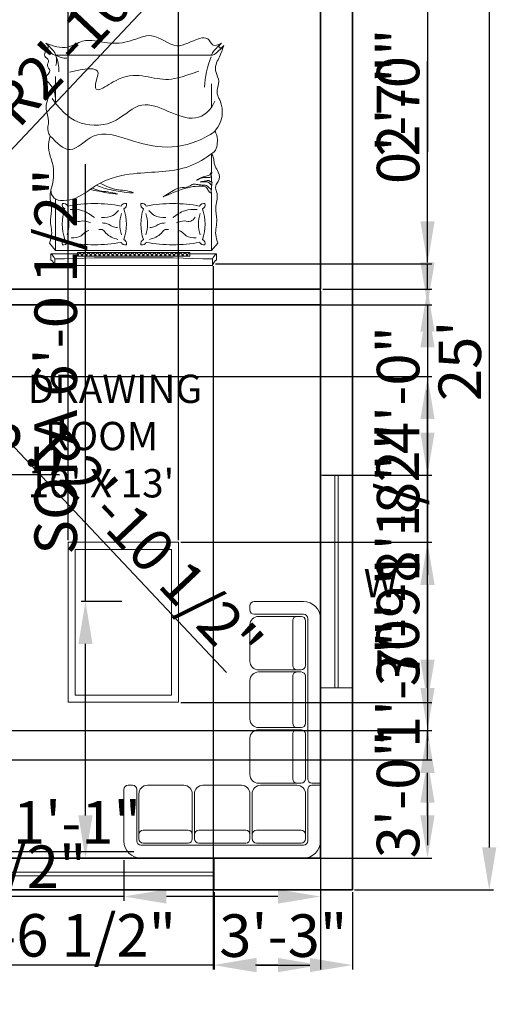
# Model space of a CAD drawing. Units: inches. Extents: x 2122 to 2726, y 1923 to 2370.
# Tile 5 of 6: x 2506 to 2641, y 1940 to 2218. Entities that reach past the tile are written whole.
import ezdxf

# ---------------------------------------------------------------- set-up
doc = ezdxf.new("R2010")
doc.units = ezdxf.units.IN
for name, color, linetype, lineweight in [('A-ANNO-DIMS', 2, 'Continuous', 18), ('A-ANNO-TEXT', 7, 'Continuous', 18), ('A-AREA-IDEN', 7, 'Continuous', 25), ('A-FURN', 8, 'Continuous', 18), ('A-GLAZ', 4, 'Continuous', 18), ('A-WALL', 7, 'Continuous', 35), ('www.cadblocksfree.com', 7, 'Continuous', 9)]:
    doc.layers.add(name, color=color, linetype=linetype, lineweight=lineweight)
doc.styles.get("Standard").update_dxf_attribs({"font": 'arial.ttf'})
doc.dimstyles.new('ISO-25', dxfattribs={"dimtxt": 12, "dimasz": 12, "dimexe": 1.25, "dimexo": 0.625, "dimtad": 1, "dimlunit": 3, "dimtxsty": 'Standard', "dimcen": 2.5, "dimadec": 0, "dimazin": 0, "dimtfac": 1, "dimtmove": 0, "dimatfit": 3, "dimfxl": 1, "dimarcsym": 0})

# ---------------------------------------------------------------- blocks, each defined once
blk = doc.blocks.new('bed')
at = {"layer": 'www.cadblocksfree.com', "ltscale": 0.2}
h = blk.add_hatch(dxfattribs=at)
h.set_pattern_fill('ANSI37,_O', color=256, scale=0.393701)
h.set_pattern_definition([(45, (2420.7222, -262.9689), (-0.8838835, 0.8838835), []), (135, (2420.7222, -262.9689), (-0.8838835, -0.8838835), [])])
h.paths.add_polyline_path([(3417.57, 1472.4), (3372.19, 1472.4), (3372.19, 1470.94), (3417.57, 1470.94)])
for p, q in [((3363, 1473.59), (3363, 1476.25)), ((3426.76, 1473.59), (3426.76, 1476.25)), ((3363.39, 1470.15), (3360.88, 1467.22)), ((3372.19, 1472.4), (3417.57, 1472.4)), ((3372.19, 1470.94), (3372.19, 1472.4)), ((3372.19, 1470.94), (3417.57, 1470.94)), ((3417.57, 1470.94), (3417.57, 1472.4)), ((3426.38, 1470.15), (3428.88, 1467.22)), ((3409.94, 1443.85), (3408.41, 1442.96)), ((3363.39, 1412.3), (3363.39, 1402.94)), ((3426.38, 1399.91), (3426.38, 1410.81)), ((3363.39, 1391.41), (3426.38, 1391.41))]:
    blk.add_line(p, q, dxfattribs=at)
for points in [[(3426.76, 1476.25), (3363, 1476.25)], [(3361.42, 1473.89), (3361.42, 1471.52), (3372.19, 1471.52)], [(3426.38, 1449.41), (3426.38, 1470.15), (3363.39, 1470.15), (3363.39, 1447.08)], [(3417.57, 1471.52), (3428.35, 1471.52), (3428.35, 1473.89)], [(3363.39, 1445.54), (3363.39, 1443.89)], [(3363.39, 1442.49), (3363.39, 1440.37)], [(3363.39, 1438.56), (3363.39, 1431.14)]]:
    blk.add_lwpolyline(points, dxfattribs=at)
for centre, radius, start, end in [((3359.33, 1477), 3.74, 303.8271, 348.4775), ((3430.43, 1477), 3.74, 191.5225, 236.1729), ((3359.84, 1474.37), 3.25, 298.9176, 345.9939), ((3394.88, 2431.36), 958.3, 268.09356, 271.90644), ((3429.92, 1474.37), 3.25, 194.0061, 241.0824), ((3367.9, 1467.4), 1.87, 165.5166, 244.2099), ((3366.56, 1466.05), 1.87, 25.7901, 104.4834), ((3379.01, 1409.19), 58.68, 79.4235, 100.5765), ((3391.47, 1466.05), 1.87, 75.5166, 154.2099), ((3390.12, 1467.4), 1.87, 295.7901, 14.4834), ((3399.64, 1467.4), 1.87, 165.5166, 244.2099), ((3398.3, 1466.05), 1.87, 25.7901, 104.4834), ((3410.75, 1409.19), 58.68, 79.4235, 100.5765), ((3423.21, 1466.05), 1.87, 75.5166, 154.2099), ((3421.86, 1467.4), 1.87, 295.7901, 14.4834), ((3385.29, 1459.55), 19.22, 161.2852, 198.7148), ((3355.42, 1459.55), 13.34, 341.1598, 18.8402), ((3402.61, 1459.55), 13.34, 161.1598, 198.8402), ((3372.74, 1459.55), 19.22, 341.2852, 18.7148), ((3417.03, 1459.55), 19.22, 161.2852, 198.7148), ((3387.15, 1459.55), 13.34, 341.1598, 18.8402), ((3434.35, 1459.55), 13.34, 161.1598, 198.8402), ((3404.48, 1459.55), 19.22, 341.2852, 18.7148), ((3367.9, 1451.7), 1.87, 115.7901, 194.4834), ((3366.56, 1453.04), 1.87, 255.5166, 334.2099), ((3379.01, 1509.91), 58.68, 259.4235, 280.5765), ((3391.47, 1453.04), 1.87, 205.7901, 284.4834), ((3390.12, 1451.7), 1.87, 345.5166, 64.2099), ((3399.64, 1451.7), 1.87, 115.7901, 194.4834), ((3398.3, 1453.04), 1.87, 255.5166, 334.2099), ((3410.75, 1509.91), 58.68, 259.4235, 280.5765), ((3423.21, 1453.04), 1.87, 205.7901, 284.4834), ((3421.86, 1451.7), 1.87, 345.5166, 64.2099), ((3424.34, 1446.05), 3.94, 342.0511, 87.9851), ((3445.78, 1439.1), 18.6, 162.0511, 198.5657), ((3365.21, 1427.6), 3.94, 125.4209, 169.6982), ((3416.57, 1428.08), 12.65, 341.0268, 23.7782), ((3370.55, 1414.19), 11.47, 139.4648, 203.3712), ((3367.28, 1412.87), 7.94, 204.0179, 212.619), ((3331.91, 1405.56), 34.38, 336.8495, 357.9003), ((3438.82, 1397.31), 13.77, 176.7525, 205.373), ((3432.14, 1393.64), 6.17, 162.6475, 201.1361), ((3422.11, 1384.8), 7.8, 58.0013, 91.6551)]:
    blk.add_arc(centre, radius, start, end, dxfattribs=at)
at = {"layer": 'www.cadblocksfree.com', "ltscale": 0.2, "extrusion": (0, 0, -1)}
for centre, major_axis, ratio, start_param, end_param in [((3360.34, 1388.37), (3.04, 3.04), 0.168252, 4.250342, 8.316029), ((3359.29, 1387.32), (1.05, 1.05), 0.453532, 4.422107, 8.144264)]:
    blk.add_ellipse(centre, major_axis=major_axis, ratio=ratio, start_param=start_param, end_param=end_param, dxfattribs=at)
at = {"layer": 'www.cadblocksfree.com', "ltscale": 0.2}
for centre, major_axis, ratio, start_param, end_param in [((3429.42, 1388.37), (-3.04, 3.04), 0.168252, 4.250342, 8.316029), ((3430.48, 1387.32), (-1.05, 1.05), 0.453532, 4.422107, 8.144264)]:
    blk.add_ellipse(centre, major_axis=major_axis, ratio=ratio, start_param=start_param, end_param=end_param, dxfattribs=at)
for points, knots in [([(3360.88, 1467.22), (3361.27, 1466.08), (3362.33, 1462.98), (3360.73, 1458.15), (3362.39, 1452.62), (3360.35, 1448.14), (3362.43, 1444.24), (3360.04, 1441.93), (3360.26, 1438.68), (3362.05, 1436.55), (3362.42, 1434.52), (3362.57, 1432.76), (3363.1, 1431.71), (3363.39, 1431.14)], [0, 0, 0, 0, 3.550403, 9.643115, 14.356056, 20.206026, 23.427697, 25.46537, 29.172767, 31.884544, 33.668442, 35.237641, 37.145618, 37.145618, 37.145618, 37.145618]), ([(3428.88, 1467.22), (3428.49, 1466.08), (3427.44, 1462.98), (3429.04, 1458.15), (3427.38, 1452.62), (3429.08, 1448.87), (3428.37, 1446.52), (3428.27, 1446.19)], [0, 0, 0, 0, 0.0901802, 0.2449351, 0.3646438, 0.5132331, 0.5378548, 0.5378548, 0.5378548, 0.5378548]), ([(3369.63, 1465.08), (3371.1, 1465.04), (3373.63, 1464.97), (3375.26, 1462.52), (3376.48, 1462.17), (3376.75, 1462.09)], [0, 0, 0, 0, 4.163459, 7.093919, 7.934624, 7.934624, 7.934624, 7.934624]), ([(3388.54, 1465.74), (3386.72, 1465.16), (3384.36, 1464.41), (3382.68, 1461.63), (3381.45, 1461.64), (3380.81, 1461.64)], [0, 0, 0, 0, 5.530688, 7.154877, 8.940839, 8.940839, 8.940839, 8.940839]), ([(3401.22, 1465.74), (3403.05, 1465.16), (3405.41, 1464.41), (3407.09, 1461.63), (3408.31, 1461.64), (3408.95, 1461.64)], [0, 0, 0, 0, 5.530688, 7.154877, 8.940839, 8.940839, 8.940839, 8.940839]), ([(3420.14, 1465.08), (3418.66, 1465.04), (3416.14, 1464.97), (3414.5, 1462.52), (3413.28, 1462.17), (3413.01, 1462.09)], [0, 0, 0, 0, 4.163459, 7.093919, 7.934624, 7.934624, 7.934624, 7.934624]), ([(3370.05, 1456.77), (3370.59, 1457.46), (3371.71, 1458.88), (3374.68, 1457.89), (3376.51, 1458.59), (3377.52, 1458.99)], [0, 0, 0, 0, 2.388143, 4.935423, 8.166198, 8.166198, 8.166198, 8.166198]), ([(3388.36, 1460.93), (3387.64, 1460.85), (3386.25, 1460.69), (3384.48, 1459.22), (3382.96, 1459.13), (3382.11, 1459.07)], [0, 0, 0, 0, 2.127543, 4.10272, 6.58647, 6.58647, 6.58647, 6.58647]), ([(3401.41, 1460.93), (3402.13, 1460.85), (3403.51, 1460.69), (3405.28, 1459.22), (3406.81, 1459.13), (3407.65, 1459.07)], [0, 0, 0, 0, 2.127543, 4.10272, 6.58647, 6.58647, 6.58647, 6.58647]), ([(3419.72, 1456.77), (3419.17, 1457.46), (3418.05, 1458.88), (3415.08, 1457.89), (3413.26, 1458.59), (3412.24, 1458.99)], [0, 0, 0, 0, 2.388143, 4.935423, 8.166198, 8.166198, 8.166198, 8.166198]), ([(3369.29, 1453.58), (3371, 1453.6), (3374.59, 1453.64), (3377.5, 1455.76), (3379.02, 1456.87)], [0, 0, 0, 0, 5.002087, 10.507046, 10.507046, 10.507046, 10.507046]), ([(3388.77, 1454), (3388.07, 1454.76), (3386.27, 1456.73), (3383.54, 1456.81), (3381.88, 1456.86)], [0, 0, 0, 0, 3.013696, 7.735839, 7.735839, 7.735839, 7.735839]), ([(3401, 1454), (3401.7, 1454.76), (3403.5, 1456.73), (3406.22, 1456.81), (3407.88, 1456.86)], [0, 0, 0, 0, 3.013696, 7.735839, 7.735839, 7.735839, 7.735839]), ([(3420.48, 1453.58), (3418.77, 1453.6), (3415.18, 1453.64), (3412.27, 1455.76), (3410.74, 1456.87)], [0, 0, 0, 0, 5.002087, 10.507046, 10.507046, 10.507046, 10.507046]), ([(3363.39, 1447.08), (3363.43, 1446.99), (3363.53, 1446.78), (3363.73, 1446.46), (3363.51, 1446.15), (3363.66, 1445.9), (3363.56, 1445.67), (3363.44, 1445.58), (3363.39, 1445.54)], [0, 0, 0, 0, 0.293454, 0.701471, 1.003873, 1.254893, 1.47342, 1.69185, 1.69185, 1.69185, 1.69185]), ([(3363.39, 1447.08), (3363.99, 1446.78), (3365.08, 1446.12), (3365.12, 1444.37), (3367.13, 1444.19), (3367.27, 1444.2)], [0.0122268, 0.0122268, 0.0122268, 0.0122268, 0.0594721, 0.1062177, 0.134458, 0.134458, 0.134458, 0.134458]), ([(3367.27, 1444.2), (3369.57, 1444.23), (3373.92, 1444.28), (3385.47, 1449.8), (3379.56, 1446.49), (3376.81, 1444.48), (3372.95, 1444.92), (3370.93, 1443.14), (3368.77, 1443.7), (3367.36, 1443.75), (3366.55, 1443.78)], [0, 0, 0, 0, 8.61026, 16.221274, 18.843057, 23.804898, 27.440828, 29.356102, 31.203478, 33.650687, 33.650687, 33.650687, 33.650687]), ([(3409.94, 1443.85), (3408.47, 1444.45), (3404.44, 1446.04), (3391.4, 1447.6), (3398.64, 1445.77), (3402.97, 1445.76), (3406.22, 1444.09), (3408.41, 1442.96)], [0.0056315, 0.0056315, 0.0056315, 0.0056315, 0.1489731, 0.3882761, 0.4793617, 0.5593494, 0.7397317, 0.7397317, 0.7397317, 0.7397317]), ([(3412.4, 1445.5), (3411.61, 1445.7), (3406.24, 1446.93), (3398.17, 1447.93), (3405.4, 1446.46), (3408.57, 1446.19), (3410.63, 1445.46), (3411.68, 1445)], [0.1043639, 0.1043639, 0.1043639, 0.1043639, 0.1489731, 0.3882761, 0.4793617, 0.5593494, 0.6446217, 0.6446217, 0.6446217, 0.6446217]), ([(3409.94, 1443.85), (3413.12, 1445.84), (3417.43, 1449.66), (3422.72, 1450.04), (3424.48, 1449.98)], [1.3582378, 1.3582378, 1.3582378, 1.3582378, 1.6381418, 1.7706953, 1.7706953, 1.7706953, 1.7706953]), ([(3362.93, 1430.81), (3365.94, 1432.96), (3375.45, 1438.99), (3392.12, 1438.03), (3404.25, 1440.73), (3408.41, 1442.96)], [0.102872, 0.102872, 0.102872, 0.102872, 0.37972, 0.957702, 1.313793, 1.313793, 1.313793, 1.313793]), ([(3363.39, 1443.89), (3363.33, 1443.81), (3363.17, 1443.56), (3363.35, 1443.12), (3363.23, 1442.79), (3363.23, 1442.53), (3363.34, 1442.51), (3363.39, 1442.49)], [0, 0, 0, 0, 0.27176, 0.887321, 1.189132, 1.388142, 1.515331, 1.515331, 1.515331, 1.515331]), ([(3366.55, 1443.78), (3366.17, 1443.78), (3365.17, 1443.9), (3364.4, 1444.96), (3363.63, 1445.46), (3363.39, 1445.54)], [0.15648839, 0.15648839, 0.15648839, 0.15648839, 0.18439755, 0.23137648, 0.25059846, 0.25059846, 0.25059846, 0.25059846]), ([(3363.39, 1443.89), (3363.63, 1443.61), (3364.67, 1442.73), (3364.89, 1442.15), (3369.07, 1442.74), (3366.77, 1442.24), (3365.83, 1442.3), (3364.61, 1441.55), (3363.96, 1442.54), (3363.54, 1442.52), (3363.39, 1442.49)], [0.0595743, 0.0595743, 0.0595743, 0.0595743, 0.0807529, 0.1037415, 0.1697201, 0.1760361, 0.2071372, 0.2404744, 0.2623409, 0.2736605, 0.2736605, 0.2736605, 0.2736605]), ([(3363.39, 1440.37), (3363.44, 1440.27), (3363.57, 1440.06), (3363.61, 1439.68), (3363.53, 1439.31), (3363.41, 1439), (3363.33, 1438.75), (3363.37, 1438.61), (3363.39, 1438.56)], [0, 0, 0, 0, 0.329977, 0.725302, 1.129072, 1.442831, 1.734218, 1.878348, 1.878348, 1.878348, 1.878348]), ([(3363.39, 1440.37), (3363.63, 1440.51), (3364.53, 1440.9), (3366.48, 1440.25), (3370.2, 1442.29), (3367.73, 1440.64), (3365.42, 1440.07), (3364.04, 1439.91), (3363.8, 1438.94), (3363.48, 1438.64), (3363.39, 1438.56)], [0.013856, 0.013856, 0.013856, 0.013856, 0.0348738, 0.0888667, 0.1078792, 0.1267378, 0.158714, 0.1937575, 0.2174868, 0.2267221, 0.2267221, 0.2267221, 0.2267221]), ([(3361.34, 1428.31), (3361.33, 1428.3), (3361.16, 1427.34), (3360.78, 1425.17), (3361.47, 1423.14), (3362.01, 1421.85)], [0.3128349, 0.3128349, 0.3128349, 0.3128349, 0.313751, 0.386958, 0.4759027, 0.4759027, 0.4759027, 0.4759027]), ([(3365.51, 1424.21), (3370.52, 1427), (3381.15, 1429.83), (3396.21, 1425.87), (3410.54, 1420.65), (3420.27, 1432.69), (3425.88, 1426.77), (3428.53, 1423.97)], [0.099185, 0.099185, 0.099185, 0.099185, 0.523647, 0.927087, 1.289918, 1.564439, 1.810555, 1.810555, 1.810555, 1.810555]), ([(3428.53, 1423.97), (3428.91, 1423.4), (3430.1, 1421.61), (3428.49, 1417.66), (3430.59, 1413.79), (3429.8, 1409.12), (3428.4, 1406.56), (3427.36, 1404.97)], [0, 0, 0, 0, 0.050513, 0.157399, 0.2842023, 0.3628173, 0.5066917, 0.5066917, 0.5066917, 0.5066917]), ([(3362.06, 1409.87), (3363.64, 1413.65), (3372.98, 1421.34), (3389.68, 1406.04), (3402.4, 1419.98), (3416.04, 1420.17), (3423.23, 1415.23), (3427.83, 1408.9)], [0.029901, 0.029901, 0.029901, 0.029901, 0.276967, 0.797115, 1.093669, 1.464666, 1.788489, 1.788489, 1.788489, 1.788489]), ([(3431.24, 1387.47), (3430.88, 1388.17), (3430.2, 1389.5), (3431.48, 1391.99), (3428.29, 1393.19), (3430.5, 1395.69), (3427.56, 1397.87), (3431.84, 1400.39), (3426.54, 1404.33), (3426.44, 1408.15), (3426.38, 1410.81)], [0, 0, 0, 0, 2.267059, 4.324559, 6.685584, 8.878641, 11.121502, 14.300359, 17.755284, 25.682856, 25.682856, 25.682856, 25.682856]), ([(3358.53, 1387.47), (3359.1, 1389.21), (3359.96, 1391.82), (3361.92, 1395.15), (3361.9, 1398.55), (3359.88, 1401.84), (3361.56, 1405.21), (3361.03, 1407.51), (3360.64, 1408.47), (3360.59, 1408.59)], [0, 0, 0, 0, 0.138875, 0.2092702, 0.2901949, 0.3858479, 0.4804923, 0.5489252, 0.5590752, 0.5590752, 0.5590752, 0.5590752]), ([(3368.63, 1397.84), (3375.98, 1400.49), (3385.35, 1402.76), (3397.53, 1395.27), (3413.59, 1410.38), (3407.81, 1395.02), (3420.76, 1398.2)], [0.029901, 0.029901, 0.029901, 0.029901, 0.276967, 0.797115, 1.093669, 1.16836, 1.16836, 1.16836, 1.16836]), ([(3430.32, 1386.56), (3427.33, 1387.65), (3422.15, 1389.55), (3414.53, 1384.14), (3405.61, 1387.05), (3396.29, 1386.31), (3386.84, 1381.28), (3377.74, 1390.27), (3370.78, 1384.8), (3364.63, 1383.97), (3363.28, 1388.27), (3360.78, 1387.15), (3359.45, 1386.56)], [0, 0, 0, 0, 8.93042, 15.449194, 25.485629, 34.878505, 43.598887, 54.554403, 64.16647, 67.461673, 70.610457, 74.213583, 74.213583, 74.213583, 74.213583])]:
    blk.add_open_spline(points, degree=3, knots=knots, dxfattribs=at)
for points in [[(3361.23, 1424.04), (3361.24, 1424.04), (3361.24, 1424.04), (3361.24, 1424.04)], [(3361.84, 1421.64), (3362.35, 1422.25), (3362.87, 1422.86), (3365.51, 1424.21)]]:
    blk.add_open_spline(points, degree=3, dxfattribs=at)
blk = doc.blocks.new('A$C2AFA021D')
for p, q in [((0.8, 2.3), (0.2, 2.3)), ((0.85, 2.2), (0.85, 2.25)), ((0, 2.1), (0, 0.2)), ((0.15, 0.2), (0.15, 2.1)), ((0.175, 1.55), (0.175, 2.075)), ((0.2, 2.15), (0.8, 2.15)), ((0.225, 2.125), (0.275, 2.125)), ((0.75, 2.125), (0.275, 2.125)), ((0.325, 2.075), (0.325, 1.55)), ((0.85, 1.6), (0.85, 2.025)), ((0.275, 1.5), (0.225, 1.5)), ((0.275, 1.5), (0.75, 1.5)), ((0.175, 0.875), (0.175, 1.425)), ((0.225, 1.475), (0.275, 1.475)), ((0.75, 1.475), (0.275, 1.475)), ((0.325, 1.425), (0.325, 0.875)), ((0.85, 0.925), (0.85, 1.375)), ((0.275, 0.825), (0.225, 0.825)), ((0.275, 0.825), (0.75, 0.825)), ((0.975, 0.825), (1.4, 0.825)), ((1.625, 0.825), (2.075, 0.825)), ((2.3, 0.825), (2.725, 0.825)), ((2.9, 0.825), (2.95, 0.825)), ((0.175, 0.225), (0.175, 0.75)), ((0.225, 0.8), (0.275, 0.8)), ((0.75, 0.8), (0.275, 0.8)), ((0.325, 0.75), (0.325, 0.225)), ((0.85, 0.275), (0.85, 0.7)), ((0.875, 0.275), (0.875, 0.725)), ((1.5, 0.725), (1.5, 0.275)), ((1.525, 0.275), (1.525, 0.725)), ((2.175, 0.725), (2.175, 0.275)), ((2.2, 0.275), (2.2, 0.725)), ((2.825, 0.725), (2.825, 0.275)), ((2.85, 0.2), (2.85, 0.775)), ((3, 0.775), (3, 0.2)), ((0.875, 0.275), (0.875, 0.225)), ((1.45, 0.325), (0.925, 0.325)), ((1.5, 0.225), (1.5, 0.275)), ((1.525, 0.275), (1.525, 0.225)), ((2.125, 0.325), (1.575, 0.325)), ((2.175, 0.225), (2.175, 0.275)), ((2.2, 0.275), (2.2, 0.225)), ((2.775, 0.325), (2.25, 0.325)), ((2.825, 0.225), (2.825, 0.275)), ((0.8, 0.15), (0.2, 0.15)), ((0.275, 0.175), (0.225, 0.175)), ((0.275, 0.175), (0.75, 0.175)), ((0.925, 0.175), (1.45, 0.175)), ((0.925, 0.15), (2.8, 0.15)), ((1.575, 0.175), (2.125, 0.175)), ((2.25, 0.175), (2.775, 0.175)), ((0.85, 0), (0.85, 0.1)), ((0.875, 0.1), (0.875, 0)), ((0.2, 0), (0.85, 0)), ((2.8, 0), (0.875, 0))]:
    blk.add_line(p, q)
for centre, radius, start, end in [((0.2, 2.1), 0.2, 90, 180), ((0.8, 2.25), 0.05, 0, 90), ((0.8, 2.2), 0.05, 270, 0), ((0.2, 2.1), 0.05, 90, 180), ((0.225, 2.075), 0.05, 90, 180), ((0.275, 2.075), 0.05, 0, 90), ((0.75, 2.025), 0.1, 0, 90), ((0.225, 1.55), 0.05, 180, 270), ((0.275, 1.55), 0.05, 270, 0), ((0.75, 1.6), 0.1, 270, 0), ((0.225, 1.425), 0.05, 90, 180), ((0.275, 1.425), 0.05, 0, 90), ((0.75, 1.375), 0.1, 360, 90), ((0.75, 0.925), 0.1, 270, 0), ((0.225, 0.875), 0.05, 180, 270), ((0.275, 0.875), 0.05, 270, 0), ((0.975, 0.725), 0.1, 90, 180), ((1.4, 0.725), 0.1, 0, 90), ((1.625, 0.725), 0.1, 90, 180), ((2.075, 0.725), 0.1, 0, 90), ((2.3, 0.725), 0.1, 90, 180), ((2.725, 0.725), 0.1, 0, 90), ((2.9, 0.775), 0.05, 90, 180), ((2.95, 0.775), 0.05, 0, 90), ((0.225, 0.75), 0.05, 90, 180), ((0.275, 0.75), 0.05, 0, 90), ((0.75, 0.7), 0.1, 0, 90), ((0.75, 0.275), 0.1, 270, 0), ((0.925, 0.275), 0.05, 90, 180), ((1.45, 0.275), 0.05, 360, 90), ((1.575, 0.275), 0.05, 90, 180), ((2.125, 0.275), 0.05, 360, 90), ((2.25, 0.275), 0.05, 90, 180), ((2.775, 0.275), 0.05, 360, 90), ((0.2, 0.2), 0.2, 180, 270), ((0.2, 0.2), 0.05, 180, 270), ((0.225, 0.225), 0.05, 180, 270), ((0.275, 0.225), 0.05, 270, 0), ((0.8, 0.1), 0.05, 0, 90), ((0.925, 0.225), 0.05, 180, 270), ((0.925, 0.1), 0.05, 90, 180), ((1.45, 0.225), 0.05, 270, 0), ((1.575, 0.225), 0.05, 180, 270), ((2.125, 0.225), 0.05, 270, 0), ((2.25, 0.225), 0.05, 180, 270), ((2.775, 0.225), 0.05, 270, 0), ((2.8, 0.2), 0.2, 270, 0), ((2.8, 0.2), 0.05, 270, 0)]:
    blk.add_arc(centre, radius, start, end)
blk = doc.blocks.new('*D9')
at = {"layer": 'A-ANNO-DIMS', "color": 0, "lineweight": -2, "transparency": 16777216}
for p, q in [((2600.63, 2271.24), (2639.88, 2271.24)), ((2638.63, 2259.24), (2638.63, 1984.74)), ((2600.63, 1972.74), (2639.88, 1972.74))]:
    blk.add_line(p, q, dxfattribs=at)
at = {"layer": 'A-ANNO-DIMS', "color": 0, "transparency": 16777216}
for points in [[(2636.63, 2259.24), (2640.63, 2259.24), (2638.63, 2271.24)], [(2636.63, 1984.74), (2640.63, 1984.74), (2638.63, 1972.74)]]:
    blk.add_solid(points, dxfattribs=at)
at = {"layer": 'Defpoints', "color": 0, "transparency": 16777216}
for p in [(2600.01, 2271.24), (2600.01, 1972.74), (2638.63, 1972.74)]:
    blk.add_point(p, dxfattribs=at)
at = {"layer": 'A-ANNO-DIMS', "color": 0, "transparency": 16777216, "insert": (2631.88, 2121.99), "char_height": 12, "attachment_point": 5, "rotation": 90}
blk.add_mtext("25'", dxfattribs=at)
blk = doc.blocks.new('WIN-60IN')
for p, q in [((0, 0), (0, 9)), ((60, 0), (60, 9)), ((0, 5), (60, 5)), ((0, 4), (60, 4))]:
    blk.add_line(p, q)
blk = doc.blocks.new('*D24')
at = {"layer": 'A-ANNO-DIMS', "color": 0, "lineweight": -2, "transparency": 16777216}
for p, q in [((2294.01, 2092.91), (2294.01, 2088.68)), ((2318.01, 2092.91), (2318.01, 2088.68)), ((2282.01, 2089.93), (2270.01, 2089.93)), ((2294.01, 2089.93), (2318.01, 2089.93)), ((2330.01, 2089.93), (2517.34, 2089.93))]:
    blk.add_line(p, q, dxfattribs=at)
at = {"layer": 'A-ANNO-DIMS', "color": 0, "transparency": 16777216}
for points in [[(2282.01, 2091.93), (2282.01, 2087.93), (2294.01, 2089.93)], [(2330.01, 2091.93), (2330.01, 2087.93), (2318.01, 2089.93)]]:
    blk.add_solid(points, dxfattribs=at)
at = {"layer": 'Defpoints', "color": 0, "transparency": 16777216}
for p in [(2294.01, 2093.53), (2318.01, 2093.53), (2318.01, 2089.93)]:
    blk.add_point(p, dxfattribs=at)
at = {"layer": 'A-ANNO-DIMS', "color": 0, "transparency": 16777216, "insert": (2429.67, 2096.76), "char_height": 12, "attachment_point": 5}
blk.add_mtext('DOOR LEAF 2\'-0" TYP.', dxfattribs=at)
blk = doc.blocks.new('*D34')
at = {"layer": 'A-ANNO-DIMS', "color": 0, "lineweight": -2, "transparency": 16777216}
for p, q in [((2524.67, 2054.11), (2524.67, 2177.46)), ((2534.9, 2054.11), (2523.42, 2054.11)), ((2524.67, 1993.74), (2524.67, 2042.11)), ((2534.9, 1981.74), (2523.42, 1981.74))]:
    blk.add_line(p, q, dxfattribs=at)
at = {"layer": 'A-ANNO-DIMS', "color": 0, "transparency": 16777216}
for points in [[(2522.67, 2042.11), (2526.67, 2042.11), (2524.67, 2054.11)], [(2522.67, 1993.74), (2526.67, 1993.74), (2524.67, 1981.74)]]:
    blk.add_solid(points, dxfattribs=at)
at = {"layer": 'Defpoints', "color": 0, "transparency": 16777216}
for p in [(2524.67, 2054.11), (2535.52, 2054.11), (2535.52, 1981.74)]:
    blk.add_point(p, dxfattribs=at)
at = {"layer": 'A-ANNO-DIMS', "color": 0, "transparency": 16777216, "insert": (2517.83, 2121.79), "char_height": 12, "attachment_point": 5, "rotation": 90}
blk.add_mtext('SOFA 6\'-0 1/2"', dxfattribs=at)
blk = doc.blocks.new('*D35')
at = {"layer": 'A-ANNO-DIMS', "color": 0, "lineweight": -2, "transparency": 16777216}
for p, q in [((2535.52, 1981.11), (2535.52, 1969.63)), ((2591.01, 1981.11), (2591.01, 1969.63)), ((2535.52, 1970.88), (2461.93, 1970.88)), ((2579.01, 1970.88), (2547.52, 1970.88))]:
    blk.add_line(p, q, dxfattribs=at)
at = {"layer": 'A-ANNO-DIMS', "color": 0, "transparency": 16777216}
for points in [[(2547.52, 1972.88), (2547.52, 1968.88), (2535.52, 1970.88)], [(2579.01, 1972.88), (2579.01, 1968.88), (2591.01, 1970.88)]]:
    blk.add_solid(points, dxfattribs=at)
at = {"layer": 'Defpoints', "color": 0, "transparency": 16777216}
for p in [(2535.52, 1981.74), (2591.01, 1981.74), (2535.52, 1970.88)]:
    blk.add_point(p, dxfattribs=at)
at = {"layer": 'A-ANNO-DIMS', "color": 0, "transparency": 16777216, "insert": (2492.72, 1977.71), "char_height": 12, "attachment_point": 5}
blk.add_mtext('4\'-7 1/2"', dxfattribs=at)
blk = doc.blocks.new('*D36')
at = {"layer": 'A-ANNO-DIMS', "color": 0, "lineweight": -2, "transparency": 16777216}
for p, q in [((2491.33, 2053.12), (2491.33, 2196.38)), ((2482.88, 2053.12), (2492.58, 2053.12)), ((2491.33, 2004.66), (2491.33, 2041.12)), ((2482.88, 1992.66), (2492.58, 1992.66))]:
    blk.add_line(p, q, dxfattribs=at)
at = {"layer": 'A-ANNO-DIMS', "color": 0, "transparency": 16777216}
for points in [[(2489.33, 2041.12), (2493.33, 2041.12), (2491.33, 2053.12)], [(2489.33, 2004.66), (2493.33, 2004.66), (2491.33, 1992.66)]]:
    blk.add_solid(points, dxfattribs=at)
at = {"layer": 'Defpoints', "color": 0, "transparency": 16777216}
for p in [(2482.26, 2053.12), (2491.33, 2053.12), (2482.26, 1992.66)]:
    blk.add_point(p, dxfattribs=at)
at = {"layer": 'A-ANNO-DIMS', "color": 0, "transparency": 16777216, "insert": (2484.5, 2130.75), "char_height": 12, "attachment_point": 5, "rotation": 90}
blk.add_mtext('TV UNIT 5\'-0 1/2"', dxfattribs=at)
blk = doc.blocks.new('*D37')
at = {"layer": 'A-ANNO-DIMS', "color": 0, "lineweight": -2, "transparency": 16777216}
for p, q in [((2469.15, 1992.03), (2469.15, 1982.34)), ((2482.26, 1992.03), (2482.26, 1982.34)), ((2457.15, 1983.59), (2445.15, 1983.59)), ((2469.15, 1983.59), (2482.26, 1983.59)), ((2494.26, 1983.59), (2538.28, 1983.59))]:
    blk.add_line(p, q, dxfattribs=at)
at = {"layer": 'A-ANNO-DIMS', "color": 0, "transparency": 16777216}
for points in [[(2457.15, 1985.59), (2457.15, 1981.59), (2469.15, 1983.59)], [(2494.26, 1985.59), (2494.26, 1981.59), (2482.26, 1983.59)]]:
    blk.add_solid(points, dxfattribs=at)
at = {"layer": 'Defpoints', "color": 0, "transparency": 16777216}
for p in [(2469.15, 1992.66), (2482.26, 1992.66), (2482.26, 1983.59)]:
    blk.add_point(p, dxfattribs=at)
at = {"layer": 'A-ANNO-DIMS', "color": 0, "transparency": 16777216, "insert": (2522.27, 1990.24), "char_height": 12, "attachment_point": 5}
blk.add_mtext('1\'-1"', dxfattribs=at)
blk = doc.blocks.new('*D40')
at = {"layer": 'A-ANNO-DIMS', "color": 0, "lineweight": -2, "transparency": 16777216}
for p, q in [((2362.13, 2017.74), (2622.46, 2017.74)), ((2621.21, 1993.74), (2621.21, 2005.74)), ((2362.13, 1981.74), (2622.46, 1981.74))]:
    blk.add_line(p, q, dxfattribs=at)
at = {"layer": 'A-ANNO-DIMS', "color": 0, "transparency": 16777216}
for points in [[(2619.21, 2005.74), (2623.21, 2005.74), (2621.21, 2017.74)], [(2619.21, 1993.74), (2623.21, 1993.74), (2621.21, 1981.74)]]:
    blk.add_solid(points, dxfattribs=at)
at = {"layer": 'Defpoints', "color": 0, "transparency": 16777216}
for p in [(2361.51, 2017.74), (2621.21, 2017.74), (2361.51, 1981.74)]:
    blk.add_point(p, dxfattribs=at)
at = {"layer": 'A-ANNO-DIMS', "color": 0, "transparency": 16777216, "insert": (2614.45, 1999.74), "char_height": 12, "attachment_point": 5, "rotation": 90}
blk.add_mtext('3\'-0"', dxfattribs=at)
blk = doc.blocks.new('*D46')
at = {"layer": 'A-ANNO-DIMS', "color": 0, "lineweight": -2, "transparency": 16777216}
for p, q in [((2591.63, 2137.74), (2622.46, 2137.74)), ((2621.21, 2125.74), (2621.21, 2101.74)), ((2591.63, 2089.74), (2622.46, 2089.74))]:
    blk.add_line(p, q, dxfattribs=at)
at = {"layer": 'A-ANNO-DIMS', "color": 0, "transparency": 16777216}
for points in [[(2619.21, 2125.74), (2623.21, 2125.74), (2621.21, 2137.74)], [(2619.21, 2101.74), (2623.21, 2101.74), (2621.21, 2089.74)]]:
    blk.add_solid(points, dxfattribs=at)
at = {"layer": 'Defpoints', "color": 0, "transparency": 16777216}
for p in [(2591.01, 2137.74), (2591.01, 2089.74), (2621.21, 2089.74)]:
    blk.add_point(p, dxfattribs=at)
at = {"layer": 'A-ANNO-DIMS', "color": 0, "transparency": 16777216, "insert": (2614.46, 2113.74), "char_height": 12, "attachment_point": 5, "rotation": 90}
blk.add_mtext('4\'-0"', dxfattribs=at)
blk = doc.blocks.new('*D47')
at = {"layer": 'A-ANNO-DIMS', "color": 0, "lineweight": -2, "transparency": 16777216}
for p, q in [((2561.01, 1972.11), (2561.01, 1950.29)), ((2600.01, 1972.11), (2600.01, 1950.29)), ((2573.01, 1951.54), (2588.01, 1951.54))]:
    blk.add_line(p, q, dxfattribs=at)
at = {"layer": 'A-ANNO-DIMS', "color": 0, "transparency": 16777216}
for points in [[(2573.01, 1953.54), (2573.01, 1949.54), (2561.01, 1951.54)], [(2588.01, 1953.54), (2588.01, 1949.54), (2600.01, 1951.54)]]:
    blk.add_solid(points, dxfattribs=at)
at = {"layer": 'Defpoints', "color": 0, "transparency": 16777216}
for p in [(2561.01, 1972.74), (2600.01, 1972.74), (2600.01, 1951.54)]:
    blk.add_point(p, dxfattribs=at)
at = {"layer": 'A-ANNO-DIMS', "color": 0, "transparency": 16777216, "insert": (2580.51, 1958.29), "char_height": 12, "attachment_point": 5}
blk.add_mtext('3\'-3"', dxfattribs=at)
blk = doc.blocks.new('*D48')
at = {"layer": 'A-ANNO-DIMS', "color": 0, "lineweight": -2, "transparency": 16777216}
for p, q in [((2519.81, 2071.41), (2519.81, 2293.69)), ((2531.81, 2292.44), (2538.94, 2292.44)), ((2550.94, 2071.41), (2550.94, 2293.69)), ((2550.94, 2292.44), (2596.29, 2292.44))]:
    blk.add_line(p, q, dxfattribs=at)
at = {"layer": 'A-ANNO-DIMS', "color": 0, "transparency": 16777216}
for points in [[(2531.81, 2294.44), (2531.81, 2290.44), (2519.81, 2292.44)], [(2538.94, 2294.44), (2538.94, 2290.44), (2550.94, 2292.44)]]:
    blk.add_solid(points, dxfattribs=at)
at = {"layer": 'Defpoints', "color": 0, "transparency": 16777216}
for p in [(2550.94, 2292.44), (2519.81, 2070.79), (2550.94, 2070.79)]:
    blk.add_point(p, dxfattribs=at)
at = {"layer": 'A-ANNO-DIMS', "color": 0, "transparency": 16777216, "insert": (2579.61, 2299.09), "char_height": 12, "attachment_point": 5}
blk.add_mtext('2\'-7"', dxfattribs=at)
blk = doc.blocks.new('*D49')
at = {"layer": 'A-ANNO-DIMS', "color": 0, "lineweight": -2, "transparency": 16777216}
for p, q in [((2551.56, 2070.79), (2622.46, 2070.79)), ((2621.21, 2058.79), (2621.21, 2037.65)), ((2551.56, 2025.65), (2622.46, 2025.65))]:
    blk.add_line(p, q, dxfattribs=at)
at = {"layer": 'A-ANNO-DIMS', "color": 0, "transparency": 16777216}
for points in [[(2619.21, 2058.79), (2623.21, 2058.79), (2621.21, 2070.79)], [(2619.21, 2037.65), (2623.21, 2037.65), (2621.21, 2025.65)]]:
    blk.add_solid(points, dxfattribs=at)
at = {"layer": 'Defpoints', "color": 0, "transparency": 16777216}
for p in [(2550.94, 2070.79), (2550.94, 2025.65), (2621.21, 2025.65)]:
    blk.add_point(p, dxfattribs=at)
at = {"layer": 'A-ANNO-DIMS', "color": 0, "transparency": 16777216, "insert": (2614.45, 2048.22), "char_height": 12, "attachment_point": 5, "rotation": 90}
blk.add_mtext('3\'-9"', dxfattribs=at)
blk = doc.blocks.new('*D52')
at = {"layer": 'A-ANNO-DIMS', "color": 0, "lineweight": -2, "transparency": 16777216}
for p, q in [((2621.21, 2149.74), (2621.21, 2161.74)), ((2314.13, 2137.74), (2622.46, 2137.74)), ((2621.21, 2137.74), (2621.21, 2117.53)), ((2314.13, 2117.53), (2622.46, 2117.53)), ((2621.21, 2105.53), (2621.21, 2061.51))]:
    blk.add_line(p, q, dxfattribs=at)
at = {"layer": 'A-ANNO-DIMS', "color": 0, "transparency": 16777216}
for points in [[(2619.21, 2149.74), (2623.21, 2149.74), (2621.21, 2137.74)], [(2619.21, 2105.53), (2623.21, 2105.53), (2621.21, 2117.53)]]:
    blk.add_solid(points, dxfattribs=at)
at = {"layer": 'Defpoints', "color": 0, "transparency": 16777216}
for p in [(2313.51, 2137.74), (2313.51, 2117.53), (2621.21, 2117.53)]:
    blk.add_point(p, dxfattribs=at)
at = {"layer": 'A-ANNO-DIMS', "color": 0, "transparency": 16777216, "insert": (2614.46, 2077.52), "char_height": 12, "attachment_point": 5, "rotation": 90}
blk.add_mtext('1\'-8"', dxfattribs=at)
blk = doc.blocks.new('*D56')
at = {"layer": 'A-ANNO-DIMS', "color": 0, "lineweight": -2, "transparency": 16777216}
for p, q in [((2621.21, 2029.74), (2621.21, 2102.85)), ((2362.13, 2017.74), (2622.46, 2017.74)), ((2621.21, 2009.39), (2621.21, 2017.74)), ((2345.6, 2009.39), (2622.46, 2009.39)), ((2621.21, 1997.39), (2621.21, 1985.39))]:
    blk.add_line(p, q, dxfattribs=at)
at = {"layer": 'A-ANNO-DIMS', "color": 0, "transparency": 16777216}
for points in [[(2619.21, 2029.74), (2623.21, 2029.74), (2621.21, 2017.74)], [(2619.21, 1997.39), (2623.21, 1997.39), (2621.21, 2009.39)]]:
    blk.add_solid(points, dxfattribs=at)
at = {"layer": 'Defpoints', "color": 0, "transparency": 16777216}
for p in [(2361.51, 2017.74), (2621.21, 2017.74), (2344.97, 2009.39)]:
    blk.add_point(p, dxfattribs=at)
at = {"layer": 'A-ANNO-DIMS', "color": 0, "transparency": 16777216, "insert": (2614.38, 2072.29), "char_height": 12, "attachment_point": 5, "rotation": 90}
blk.add_mtext('0\'-8 1/2"', dxfattribs=at)
blk = doc.blocks.new('*D57')
at = {"layer": 'A-ANNO-DIMS', "color": 0, "lineweight": -2, "transparency": 16777216}
for p, q in [((2550.94, 2071.41), (2550.94, 2293.69)), ((2579.01, 2292.44), (2562.94, 2292.44)), ((2591.01, 2090.36), (2591.01, 2293.69))]:
    blk.add_line(p, q, dxfattribs=at)
at = {"layer": 'A-ANNO-DIMS', "color": 0, "transparency": 16777216}
for points in [[(2562.94, 2294.44), (2562.94, 2290.44), (2550.94, 2292.44)], [(2579.01, 2294.44), (2579.01, 2290.44), (2591.01, 2292.44)]]:
    blk.add_solid(points, dxfattribs=at)
at = {"layer": 'Defpoints', "color": 0, "transparency": 16777216}
for p in [(2550.94, 2292.44), (2591.01, 2089.74), (2550.94, 2070.79)]:
    blk.add_point(p, dxfattribs=at)
at = {"layer": 'A-ANNO-DIMS', "color": 0, "transparency": 16777216, "insert": (2570.97, 2299.19), "char_height": 12, "attachment_point": 5}
blk.add_mtext('3\'-4"', dxfattribs=at)
blk = doc.blocks.new('*D58')
at = {"layer": 'A-ANNO-DIMS', "color": 0, "lineweight": -2, "transparency": 16777216}
for p, q in [((2621.21, 2101.74), (2621.21, 2113.74)), ((2591.63, 2089.74), (2622.46, 2089.74)), ((2621.21, 2089.74), (2621.21, 2070.79)), ((2551.56, 2070.79), (2622.46, 2070.79)), ((2621.21, 2058.79), (2621.21, 2014.77))]:
    blk.add_line(p, q, dxfattribs=at)
at = {"layer": 'A-ANNO-DIMS', "color": 0, "transparency": 16777216}
for points in [[(2619.21, 2101.74), (2623.21, 2101.74), (2621.21, 2089.74)], [(2619.21, 2058.79), (2623.21, 2058.79), (2621.21, 2070.79)]]:
    blk.add_solid(points, dxfattribs=at)
at = {"layer": 'Defpoints', "color": 0, "transparency": 16777216}
for p in [(2591.01, 2089.74), (2550.94, 2070.79), (2621.21, 2070.79)]:
    blk.add_point(p, dxfattribs=at)
at = {"layer": 'A-ANNO-DIMS', "color": 0, "transparency": 16777216, "insert": (2614.56, 2030.78), "char_height": 12, "attachment_point": 5, "rotation": 90}
blk.add_mtext('1\'-7"', dxfattribs=at)
blk = doc.blocks.new('*D62')
at = {"layer": 'A-ANNO-DIMS', "color": 0, "lineweight": -2, "transparency": 16777216}
for p, q in [((2560.71, 2148.71), (2560.71, 1950.29)), ((2591.01, 2141.61), (2591.01, 1950.29)), ((2560.71, 1951.54), (2487.39, 1951.54)), ((2579.01, 1951.54), (2572.71, 1951.54))]:
    blk.add_line(p, q, dxfattribs=at)
at = {"layer": 'A-ANNO-DIMS', "color": 0, "transparency": 16777216}
for points in [[(2572.71, 1953.54), (2572.71, 1949.54), (2560.71, 1951.54)], [(2579.01, 1953.54), (2579.01, 1949.54), (2591.01, 1951.54)]]:
    blk.add_solid(points, dxfattribs=at)
at = {"layer": 'Defpoints', "color": 0, "transparency": 16777216}
for p in [(2560.71, 2149.34), (2591.01, 2142.24), (2560.71, 1951.54)]:
    blk.add_point(p, dxfattribs=at)
at = {"layer": 'A-ANNO-DIMS', "color": 0, "transparency": 16777216, "insert": (2518.05, 1958.37), "char_height": 12, "attachment_point": 5}
blk.add_mtext('2\'-6 1/2"', dxfattribs=at)
blk = doc.blocks.new('*D63')
at = {"layer": 'A-ANNO-DIMS', "color": 0, "lineweight": -2, "transparency": 16777216}
for p, q in [((2621.21, 2161.34), (2621.21, 2206.49)), ((2561.34, 2149.34), (2622.46, 2149.34)), ((2621.21, 2142.24), (2621.21, 2149.34)), ((2591.63, 2142.24), (2622.46, 2142.24)), ((2621.21, 2130.24), (2621.21, 2118.24))]:
    blk.add_line(p, q, dxfattribs=at)
at = {"layer": 'A-ANNO-DIMS', "color": 0, "transparency": 16777216}
for points in [[(2619.21, 2161.34), (2623.21, 2161.34), (2621.21, 2149.34)], [(2619.21, 2130.24), (2623.21, 2130.24), (2621.21, 2142.24)]]:
    blk.add_solid(points, dxfattribs=at)
at = {"layer": 'Defpoints', "color": 0, "transparency": 16777216}
for p in [(2560.71, 2149.34), (2621.21, 2149.34), (2591.01, 2142.24)]:
    blk.add_point(p, dxfattribs=at)
at = {"layer": 'A-ANNO-DIMS', "color": 0, "transparency": 16777216, "insert": (2614.46, 2189.91), "char_height": 12, "attachment_point": 5, "rotation": 90}
blk.add_mtext('0\'-7"', dxfattribs=at)
blk = doc.blocks.new('*D67')
at = {"layer": 'A-ANNO-DIMS', "color": 0, "lineweight": -2, "transparency": 16777216}
for p, q in [((2621.21, 2274.24), (2621.21, 2286.24)), ((2467.13, 2262.24), (2622.46, 2262.24)), ((2621.21, 2262.24), (2621.21, 2238.32)), ((2461.84, 2238.32), (2622.46, 2238.32)), ((2621.21, 2226.32), (2621.21, 2180.97))]:
    blk.add_line(p, q, dxfattribs=at)
at = {"layer": 'A-ANNO-DIMS', "color": 0, "transparency": 16777216}
for points in [[(2619.21, 2274.24), (2623.21, 2274.24), (2621.21, 2262.24)], [(2619.21, 2226.32), (2623.21, 2226.32), (2621.21, 2238.32)]]:
    blk.add_solid(points, dxfattribs=at)
at = {"layer": 'Defpoints', "color": 0, "transparency": 16777216}
for p in [(2466.51, 2262.24), (2461.22, 2238.32), (2621.21, 2238.32)]:
    blk.add_point(p, dxfattribs=at)
at = {"layer": 'A-ANNO-DIMS', "color": 0, "transparency": 16777216, "insert": (2614.46, 2197.64), "char_height": 12, "attachment_point": 5, "rotation": 90}
blk.add_mtext('2\'-0"', dxfattribs=at)
blk = doc.blocks.new('*D71')
at = {"layer": 'A-ANNO-DIMS', "color": 0, "lineweight": -2, "transparency": 16777216}
for p, q in [((2564.44, 2245.87), (2499.95, 2177.59)), ((2468.06, 2143.82), (2491.71, 2168.87))]:
    blk.add_line(p, q, dxfattribs=at)
at = {"layer": 'A-ANNO-DIMS', "color": 0, "transparency": 16777216}
blk.add_solid([(2498.5, 2178.96), (2501.41, 2176.22), (2491.71, 2168.87)], dxfattribs=at)
at = {"layer": 'Defpoints', "color": 0, "transparency": 16777216}
for p in [(2491.71, 2168.87), (2468.06, 2143.82)]:
    blk.add_point(p, dxfattribs=at)
at = {"layer": 'A-ANNO-DIMS', "color": 0, "transparency": 16777216, "insert": (2531.35, 2220.78), "char_height": 12, "attachment_point": 5, "rotation": 46.6362}
blk.add_mtext('R2\'-10 1/2"', dxfattribs=at)
blk = doc.blocks.new('*D72')
at = {"layer": 'A-ANNO-DIMS', "color": 0, "lineweight": -2, "transparency": 16777216}
for p, q in [((2468.16, 2136.04), (2491.75, 2111.07)), ((2564.47, 2034.07), (2499.99, 2102.35))]:
    blk.add_line(p, q, dxfattribs=at)
at = {"layer": 'A-ANNO-DIMS', "color": 0, "transparency": 16777216}
blk.add_solid([(2501.44, 2103.72), (2498.53, 2100.97), (2491.75, 2111.07)], dxfattribs=at)
at = {"layer": 'Defpoints', "color": 0, "transparency": 16777216}
for p in [(2468.16, 2136.04), (2491.75, 2111.07)]:
    blk.add_point(p, dxfattribs=at)
at = {"layer": 'A-ANNO-DIMS', "color": 0, "transparency": 16777216, "insert": (2541.31, 2068.53), "char_height": 12, "attachment_point": 5, "rotation": 313.3635}
blk.add_mtext('R2\'-10 1/2"', dxfattribs=at)

msp = doc.modelspace()

# ---------------------------------------------------------------- linework, layer by layer
at = {"layer": 'A-FURN'}
for points in [[(2519.809, 2070.789), (2550.937, 2070.789), (2550.937, 2025.654), (2519.809, 2025.654)], [(2521.809, 2068.789), (2548.937, 2068.789), (2548.937, 2027.654), (2521.809, 2027.654)]]:
    msp.add_lwpolyline(points, close=True, dxfattribs=at)
at = {"layer": 'A-WALL'}
for p, q in [((2600.008, 1972.736), (2600.008, 2271.236)), ((2591.008, 2142.236), (2591.008, 2262.236)), ((2471.008, 2142.236), (2591.008, 2142.236)), ((2471.008, 2137.736), (2591.008, 2137.736)), ((2591.008, 2137.736), (2591.008, 1981.736)), ((2471.008, 1981.736), (2591.008, 1981.736)), ((2471.008, 1972.736), (2600.008, 1972.736))]:
    msp.add_line(p, q, dxfattribs=at)

# ---------------------------------------------------------------- block references
at = {"layer": 'A-FURN'}
for name, p, xscale, yscale, zscale, rotation in [('bed', (4911.58, 3180.871), 0.6990837586902172, 0.6990837586902172, 0.6990837586902172, 180), ('A$C2AFA021D', (2591.008, 1981.736), 24.12458441664085, 24.12458441664085, 24.12458441664085, 90)]:
    msp.add_blockref(name, p, dxfattribs=dict(at, xscale=xscale, yscale=yscale, zscale=zscale, rotation=rotation))
at = {"layer": 'A-GLAZ', "rotation": 270}
msp.add_blockref('WIN-60IN', (2591.008, 2089.736), dxfattribs=at)
at = {"layer": 'A-GLAZ'}
msp.add_blockref('WIN-60IN', (2501.008, 1972.736), dxfattribs=at)

# ---------------------------------------------------------------- texts
at = {"layer": 'A-ANNO-TEXT', "insert": (2603.209, 2063.25), "char_height": 7.99, "attachment_point": 1}
msp.add_mtext_dynamic_manual_height_columns('W', width=65.06795, gutter_width=39.949, heights=[0], dxfattribs=at)
at = {"layer": 'A-AREA-IDEN', "insert": (2508.369, 2118.076), "char_height": 7.9897, "attachment_point": 1}
msp.add_mtext_dynamic_manual_height_columns("DRAWING \\P  ROOM\\P10' X 13'", width=65.06795, gutter_width=39.949, heights=[0], dxfattribs=at)

# ---------------------------------------------------------------- dimensions: what is measured, and where the dimension line sits
at = {"layer": 'A-ANNO-DIMS'}
for base, p1, p2, picture, middle in [((2550.937, 2292.436), (2519.809, 2070.789), (2550.937, 2070.789), '*D48', (2579.614, 2299.086)), ((2550.937, 2292.436), (2591.008, 2089.736), (2550.937, 2070.789), '*D57', (2570.973, 2299.192)), ((2560.71, 1951.536), (2591.008, 2142.236), (2560.71, 2149.338), '*D62', (2518.053, 1958.366)), ((2482.256, 1983.587), (2469.154, 1992.656), (2482.256, 1992.656), '*D37', (2522.266, 1990.237)), ((2600.008, 1951.536), (2561.008, 1972.736), (2600.008, 1972.736), '*D47', (2580.508, 1958.292))]:
    dim = msp.add_linear_dim(base=base, p1=p1, p2=p2, dimstyle='ISO-25', override={"dimdec": 1, "dimlfac": 1, "dimrnd": 0, "dimzin": 1, "dimdsep": 46, "dimlunit": 4, "dimfrac": 2}, dxfattribs=at)
    dim.commit()
    dim.dimension.update_dxf_attribs({"geometry": picture, "text_midpoint": middle})
for base, p1, p2, angle, picture, middle in [((2621.208, 2238.321), (2466.508, 2262.236), (2461.216, 2238.321), 90, '*D67', (2614.456, 2197.644)), ((2621.208, 2149.338), (2591.008, 2142.236), (2560.71, 2149.338), 90, '*D63', (2614.456, 2189.913)), ((2621.208, 2117.531), (2313.508, 2137.736), (2313.508, 2117.531), 90, '*D52', (2614.456, 2077.521)), ((2621.208, 2089.736), (2591.008, 2137.736), (2591.008, 2089.736), 90, '*D46', (2614.456, 2113.736)), ((2621.208, 2070.789), (2591.008, 2089.736), (2550.937, 2070.789), 90, '*D58', (2614.558, 2030.779)), ((2621.208, 2017.736), (2344.971, 2009.385), (2361.508, 2017.736), 90, '*D56', (2614.378, 2072.291)), ((2621.208, 2025.654), (2550.937, 2070.789), (2550.937, 2025.654), 90, '*D49', (2614.452, 2048.221)), ((2621.208, 2017.736), (2361.508, 1981.736), (2361.508, 2017.736), 90, '*D40', (2614.452, 1999.736)), ((2535.521, 1970.88), (2591.008, 1981.736), (2535.521, 1981.736), 180, '*D35', (2492.724, 1977.71))]:
    dim = msp.add_linear_dim(base=base, p1=p1, p2=p2, angle=angle, dimstyle='ISO-25', override={"dimdec": 1, "dimlfac": 1, "dimrnd": 0, "dimzin": 1, "dimdsep": 46, "dimlunit": 4, "dimfrac": 2}, dxfattribs=at)
    dim.commit()
    dim.dimension.update_dxf_attribs({"geometry": picture, "text_midpoint": middle})
for base, p1, p2, text, override, picture, middle in [((2638.632, 1972.736), (2600.008, 2271.236), (2600.008, 1972.736), "25'", {"dimclrd": 0, "dimclre": 0, "dimclrt": 0}, '*D9', (2631.88, 2121.986)), ((2491.325, 2053.118), (2482.256, 1992.656), (2482.256, 2053.118), 'TV UNIT <>', {"dimdec": 1, "dimlfac": 1, "dimrnd": 0, "dimzin": 1, "dimdsep": 46, "dimlunit": 4, "dimfrac": 2}, '*D36', (2484.496, 2130.749)), ((2524.665, 2054.11), (2535.521, 1981.736), (2535.521, 2054.11), 'SOFA <>', {"dimdec": 1, "dimlfac": 1, "dimrnd": 0, "dimzin": 1, "dimdsep": 46, "dimlunit": 4, "dimfrac": 2}, '*D34', (2517.831, 2121.787))]:
    dim = msp.add_linear_dim(base=base, p1=p1, p2=p2, angle=90, text=text, dimstyle='ISO-25', override=override, dxfattribs=at)
    dim.commit()
    dim.dimension.update_dxf_attribs({"geometry": picture, "text_midpoint": middle})
for center, mpoint, picture, middle in [((2468.058, 2143.819), (2491.714, 2168.866), '*D71', (2531.352, 2220.781)), ((2468.165, 2136.04), (2491.746, 2111.072), '*D72', (2541.314, 2068.535))]:
    dim = msp.add_radius_dim(center=center, mpoint=mpoint, dimstyle='ISO-25', override={"dimdec": 1, "dimlfac": 1, "dimrnd": 0, "dimzin": 1, "dimdsep": 46, "dimlunit": 4, "dimfrac": 2}, dxfattribs=at)
    dim.commit()
    dim.dimension.update_dxf_attribs({"geometry": picture, "text_midpoint": middle})
dim = msp.add_linear_dim(base=(2318.008, 2089.931), p1=(2294.008, 2093.531), p2=(2318.008, 2093.531), text='DOOR LEAF <> TYP.', dimstyle='ISO-25', override={"dimdec": 1, "dimlfac": 1, "dimrnd": 0, "dimzin": 1, "dimdsep": 46, "dimlunit": 4, "dimfrac": 2}, dxfattribs=at)
dim.commit()
dim.dimension.update_dxf_attribs({"geometry": '*D24', "text_midpoint": (2429.674, 2096.764)})

doc.saveas('drawing.dxf')
